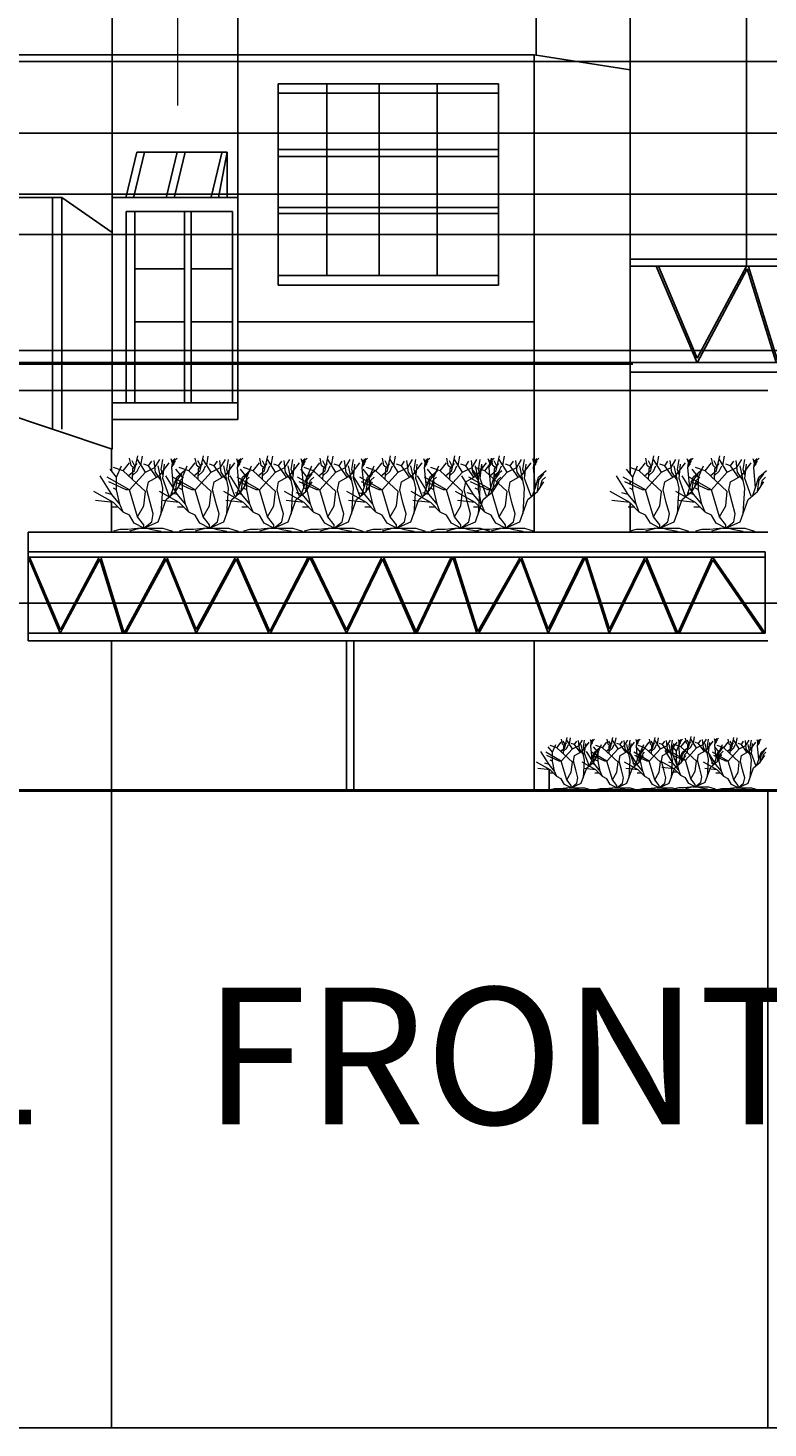
# Model space of a CAD drawing. Units: inches. Extents: x -32109 to 33221, y -19197 to 7608.
# Tile 8 of 25: x -15627 to -11787, y -5430 to 1836. Entities that reach past the tile are written whole.
import ezdxf

# ---------------------------------------------------------------- set-up
doc = ezdxf.new("R2010")
doc.units = ezdxf.units.IN
doc.header["$MEASUREMENT"] = 0
for name, color, linetype, lineweight in [('A-ANNO-DIMS', 2, 'Continuous', 18), ('A-ANNO-NOTE', 2, 'Continuous', 18), ('A-ANNO-TEXT', 7, 'Continuous', 25), ('A-ELEV', 7, 'Continuous', 25), ('L-PLNT', 3, 'Continuous', 13)]:
    doc.layers.add(name, color=color, linetype=linetype, lineweight=lineweight)
doc.styles.get("Standard").update_dxf_attribs({"font": 'arial.ttf'})
doc.dimstyles.get("Standard").update_dxf_attribs({"dimtxt": 0.18, "dimasz": 0.18, "dimexe": 0.18, "dimexo": 0.0625, "dimgap": 0.09, "dimtad": 0, "dimtih": 1, "dimtoh": 1, "dimdec": 4, "dimzin": 0, "dimdsep": 46, "dimtxsty": 'Standard', "dimcen": 0.09, "dimadec": 0, "dimazin": 0, "dimtfac": 1, "dimtdec": 4, "dimtofl": 0, "dimtmove": 0, "dimatfit": 3, "dimfxl": 1, "dimtolj": 1, "dimtzin": 0, "dimarcsym": 0})

# ---------------------------------------------------------------- blocks, each defined once
blk = doc.blocks.new('*U3')
for p, q in [((-12.47099999999977, 19.77499999999986), (-12.89799999999991, 22.04399999999987)), ((-11.27999999999997, 19.61899999999991), (-12.10400000000004, 21.18399999999974)), ((-11.43299999999999, 18.28899999999976), (-10.45699999999988, 22.7489999999998)), ((-8.160000000000082, 17.75999999999999), (-10.55999999999994, 21.59999999999991)), ((-9.480000000000018, 19.77499999999986), (-8.991999999999962, 22.59199999999964)), ((-7.200000000000045, 19.67999999999983), (-6.240000000000009, 21.11999999999989)), ((-5.085999999999785, 17.74099999999998), (-5.512999999999919, 21.33999999999992)), ((-5.279999999999972, 19.19999999999982), (-3.840000000000145, 21.59999999999991)), ((-3.376999999999952, 18.60199999999963), (-2.887999999999919, 21.57499999999982)), ((-0.5079999999998109, 21.88799999999969), (-0.0809999999999036, 20.55799999999976)), ((-0.2029999999999745, 19.14899999999988), (0.1020000000000891, 21.33999999999992)), ((-0.0199999999999818, 20.00999999999999), (0.895999999999958, 21.10499999999979)), ((0.04099999999994, 20.71399999999994), (1.384000000000241, 22.04399999999987)), ((0.1020000000000891, 21.33999999999992), (0.8350000000000363, 21.88799999999969)), ((-16.79999999999995, 16.31999999999993), (-18.7199999999998, 18.7199999999998)), ((-14.87999999999988, 18.24000000000001), (-17.75999999999999, 19.19999999999982)), ((-16.79999999999995, 16.31999999999993), (-15.3599999999999, 19.67999999999983)), ((-14.87999999999988, 18.24000000000001), (-12.95999999999981, 20.63999999999987)), ((-8.160000000000082, 12), (-14.87999999999988, 18.24000000000001)), ((-13.32499999999982, 16.72399999999993), (-11.43299999999999, 18.28899999999976)), ((-12.95999999999981, 12.47999999999979), (-8.160000000000082, 17.75999999999999)), ((-11.67699999999991, 19.07099999999991), (-12.47099999999977, 19.77499999999986)), ((-12.04299999999989, 15.6279999999997), (-11.92099999999982, 18.83600000000001)), ((-11.98199999999997, 16.80199999999968), (-10.57899999999995, 18.05399999999986)), ((-11.92099999999982, 18.83600000000001), (-10.6400000000001, 20.40100000000007)), ((-10.57899999999995, 18.05399999999986), (-9.845999999999776, 19.69699999999966)), ((-7.200000000000045, 19.67999999999983), (-8.6400000000001, 20.15999999999985)), ((-8.160000000000082, 17.75999999999999), (-5.279999999999972, 19.19999999999982)), ((-4.799999999999954, 16.31999999999993), (-7.200000000000045, 19.67999999999983)), ((-3.376999999999952, 15.31499999999982), (-5.085999999999785, 17.81899999999973)), ((-2.880000000000109, 12.95999999999981), (-4.319999999999936, 19.67999999999983)), ((-3.840000000000145, 16.79999999999995), (-0.9600000000000363, 20.63999999999987)), ((-2.765999999999849, 16.80199999999968), (-3.376999999999952, 18.60199999999963)), ((-2.880000000000109, 15.83999999999992), (-2.40000000000009, 20.15999999999985)), ((0.3460000000000036, 13.20299999999974), (-0.2029999999999745, 19.14899999999988)), ((-0.1419999999998254, 19.38399999999979), (0.5899999999999181, 20.40100000000007)), ((1.323000000000092, 16.2539999999999), (3.642000000000052, 18.28899999999976)), ((1.440000000000054, 15.3599999999999), (2.879999999999881, 17.27999999999997)), ((-18.23999999999978, 11.03999999999996), (-21.75499999999988, 16.65499999999997)), ((-12.95999999999981, 12.47999999999979), (-19.67999999999983, 16.31999999999993)), ((-13.91999999999984, 12.47999999999979), (-19.19999999999982, 14.87999999999988)), ((-16.79999999999995, 12.47999999999979), (-17.75999999999999, 12.95999999999981)), ((-16.79999999999995, 12.47999999999979), (-16.79999999999995, 16.31999999999993)), ((-7.680000000000063, 12.47999999999979), (-7.200000000000045, 14.87999999999988)), ((-7.200000000000045, 14.87999999999988), (-3.840000000000145, 16.79999999999995)), ((-3.360000000000127, 5.279999999999972), (-2.880000000000109, 12.95999999999981)), ((-0.9600000000000363, 10.55999999999994), (-2.880000000000109, 15.83999999999992)), ((-0.4800000000000182, 10.79999999999995), (0.3460000000000036, 13.20299999999974)), ((0.3460000000000036, 13.20299999999974), (1.323000000000092, 16.2539999999999)), ((0.9600000000000363, 12), (1.440000000000054, 15.3599999999999)), ((0.9600000000000363, 12), (2.879999999999881, 14.87999999999988)), ((1.920000000000072, 13.43999999999982), (2.399999999999863, 15.3599999999999)), ((2.399999999999863, 15.3599999999999), (3.359999999999899, 16.31999999999993)), ((-17.75999999999999, 8.639999999999873), (-23.66300000000001, 11.96100000000001)), ((-17.75999999999999, 8.639999999999873), (-23.12799999999993, 9.221999999999753)), ((-18.23999999999978, 11.03999999999996), (-20.15999999999985, 11.51999999999998)), ((-15.83999999999992, 8.159999999999854), (-18.23999999999978, 11.03999999999996)), ((-14.87999999999988, 5.75999999999999), (-17.75999999999999, 8.639999999999873)), ((-15.83999999999992, 8.159999999999854), (-16.79999999999995, 12.47999999999979)), ((-12.95999999999981, 12.47999999999979), (-13.91999999999984, 12.47999999999979)), ((-10.55999999999994, 4.319999999999936), (-12.95999999999981, 12.47999999999979)), ((-8.6400000000001, 7.679999999999836), (-8.160000000000082, 12)), ((-6.720000000000027, 8.639999999999873), (-7.680000000000063, 12.47999999999979)), ((-5.75999999999999, 5.279999999999972), (-6.720000000000027, 8.639999999999873)), ((-4.319999999999936, 2.879999999999881), (-1.920000000000072, 9.599999999999909)), ((-1.920000000000072, 9.599999999999909), (0.9600000000000363, 12)), ((-16.31999999999993, 7.199999999999818), (-18.23999999999978, 7.199999999999818)), ((-14.87999999999988, 5.75999999999999), (-15.83999999999992, 8.159999999999854)), ((-12.95999999999981, 4.799999999999954), (-14.87999999999988, 5.75999999999999)), ((-11.51999999999998, 2.399999999999863), (-12.95999999999981, 4.799999999999954)), ((-10.55999999999994, 4.319999999999936), (-8.6400000000001, 7.679999999999836)), ((-8.6400000000001, 1.919999999999845), (-10.55999999999994, 4.319999999999936)), ((-6.240000000000009, 2.879999999999881), (-5.75999999999999, 5.279999999999972)), ((-15.83999999999992, 0.4799999999997909), (-17.75999999999999, 0)), ((-13.43999999999982, 0.4799999999997909), (-15.83999999999992, 0.4799999999997909)), ((-9.600000000000136, 0.959999999999809), (-13.43999999999982, 0.4799999999997909)), ((-9.600000000000136, 0.959999999999809), (-12.95999999999981, 0)), ((-8.6400000000001, 0.959999999999809), (-11.51999999999998, 2.399999999999863)), ((-9.600000000000136, 0.959999999999809), (-7.680000000000063, 0.959999999999809)), ((-8.6400000000001, 0.959999999999809), (-4.319999999999936, 2.879999999999881)), ((-8.6400000000001, 0.959999999999809), (-6.240000000000009, 2.879999999999881)), ((-8.6400000000001, 0.959999999999809), (-8.6400000000001, 1.919999999999845)), ((-8.6400000000001, 0.959999999999809), (-2.880000000000109, 0.959999999999809)), ((-7.680000000000063, 0.959999999999809), (-6.240000000000009, 0.4799999999997909)), ((-6.240000000000009, 0.4799999999997909), (-3.360000000000127, 0)), ((-2.880000000000109, 0.959999999999809), (0, 0))]:
    blk.add_line(p, q)
blk = doc.blocks.new('*D10')
at = {"layer": 'A-ANNO-DIMS', "color": 0, "lineweight": -2, "transparency": 16777216}
for p, q in [((-18512.646816, -110.179138), (-18512.646816, 5772.015489000001)), ((-18512.466816, 5771.835489), (-202.0927503703958, 5771.835489)), ((18109.136745, 5771.835489), (-201.2373206296045, 5771.835489)), ((18109.316745, -101.537382), (18109.316745, 5772.015489000001))]:
    blk.add_line(p, q, dxfattribs=at)
at = {"layer": 'A-ANNO-DIMS', "color": 0, "transparency": 16777216}
for points in [[(-18512.466816, 5771.865488999999), (-18512.466816, 5771.805489000001), (-18512.646816, 5771.835489)], [(18109.136745, 5771.865488999999), (18109.136745, 5771.805489000001), (18109.316745, 5771.835489)]]:
    blk.add_solid(points, dxfattribs=at)
at = {"layer": 'Defpoints', "color": 0, "transparency": 16777216}
for p in [(18109.316745, 5771.835489), (-18512.646816, -110.241638), (18109.316745, -101.599882)]:
    blk.add_point(p, dxfattribs=at)
at = {"layer": 'A-ANNO-DIMS', "color": 0, "transparency": 16777216, "insert": (-201.6650355000002, 5771.835489), "char_height": 0.18, "attachment_point": 5}
blk.add_mtext('\\A1;36622', dxfattribs=at)
blk = doc.blocks.new('*D11')
at = {"layer": 'A-ANNO-DIMS', "color": 0, "lineweight": -2, "transparency": 16777216}
for p, q in [((14509.612941, 1705.161904000001), (25710.64858400003, 1705.161904000003)), ((25710.46858400003, 1704.981904000003), (25710.46858400003, -209.6323674706641)), ((25710.46858400003, -2124.610567999994), (25710.46858400003, -209.9962965293272)), ((-18512.58431600001, -2124.790568000001), (25710.64858400003, -2124.790567999994))]:
    blk.add_line(p, q, dxfattribs=at)
at = {"layer": 'A-ANNO-DIMS', "color": 0, "transparency": 16777216}
for points in [[(25710.43858400003, 1704.981904000003), (25710.49858400002, 1704.981904000003), (25710.46858400003, 1705.161904000003)], [(25710.43858400003, -2124.610567999994), (25710.49858400002, -2124.610567999994), (25710.46858400003, -2124.790567999994)]]:
    blk.add_solid(points, dxfattribs=at)
at = {"layer": 'Defpoints', "color": 0, "transparency": 16777216}
for p in [(14509.550441, 1705.161904000001), (-18512.64681600001, -2124.790568000001), (25710.46858400003, -2124.790567999994)]:
    blk.add_point(p, dxfattribs=at)
at = {"layer": 'A-ANNO-DIMS', "color": 0, "transparency": 16777216, "insert": (25710.46858400002, -209.8143320000029), "char_height": 0.18, "attachment_point": 5}
blk.add_mtext('\\A1;3830', dxfattribs=at)
blk = doc.blocks.new('*D21')
at = {"layer": 'A-ANNO-DIMS', "color": 0, "lineweight": -2, "transparency": 16777216}
for p, q in [((-5532.163600000002, -1149.229573), (-24361.99565300002, -1149.229573000003)), ((-24361.81565300002, -1149.409573000004), (-24361.81565300002, -1636.828167362214)), ((-24361.81565300002, -2124.610568000004), (-24361.81565300002, -1637.191973637794)), ((-5677.141660000002, -2124.790568000001), (-24361.99565300002, -2124.790568000003))]:
    blk.add_line(p, q, dxfattribs=at)
at = {"layer": 'A-ANNO-DIMS', "color": 0, "transparency": 16777216}
for points in [[(-24361.84565300001, -1149.409573000004), (-24361.78565300002, -1149.409573000004), (-24361.81565300002, -1149.229573000003)], [(-24361.84565300001, -2124.610568000004), (-24361.78565300002, -2124.610568000004), (-24361.81565300002, -2124.790568000003)]]:
    blk.add_solid(points, dxfattribs=at)
at = {"layer": 'Defpoints', "color": 0, "transparency": 16777216}
for p in [(-24361.81565300002, -1149.229573000003), (-5532.101100000001, -1149.229573), (-5677.079160000002, -2124.790568000001)]:
    blk.add_point(p, dxfattribs=at)
at = {"layer": 'A-ANNO-DIMS', "color": 0, "transparency": 16777216, "insert": (-24361.81565300001, -1637.010070499996), "char_height": 0.18, "attachment_point": 5}
blk.add_mtext('\\A1;975.6', dxfattribs=at)
blk = doc.blocks.new('*D25')
at = {"layer": 'A-ANNO-DIMS', "color": 0, "lineweight": -2, "transparency": 16777216}
for p, q in [((-15909.074234, -2124.853068), (-15909.074234, -5429.734913)), ((-15192.599186, -2124.853068), (-15192.599186, -5429.734913)), ((-15908.894234, -5429.554913), (-15551.2303525648, -5429.554913)), ((-15192.779186, -5429.554913), (-15550.4430674352, -5429.554913))]:
    blk.add_line(p, q, dxfattribs=at)
at = {"layer": 'A-ANNO-DIMS', "color": 0, "transparency": 16777216}
for points in [[(-15908.894234, -5429.524913), (-15908.894234, -5429.584913), (-15909.074234, -5429.554913)], [(-15192.779186, -5429.524913), (-15192.779186, -5429.584913), (-15192.599186, -5429.554913)]]:
    blk.add_solid(points, dxfattribs=at)
at = {"layer": 'Defpoints', "color": 0, "transparency": 16777216}
for p in [(-15909.074234, -2124.790568), (-15192.599186, -2124.790568), (-15192.599186, -5429.554913)]:
    blk.add_point(p, dxfattribs=at)
at = {"layer": 'A-ANNO-DIMS', "color": 0, "transparency": 16777216, "insert": (-15550.83671, -5429.554913), "char_height": 0.18, "attachment_point": 5}
blk.add_mtext('\\A1;716.5', dxfattribs=at)
blk = doc.blocks.new('*D26')
at = {"layer": 'A-ANNO-DIMS', "color": 0, "lineweight": -2, "transparency": 16777216}
for p, q in [((-15192.599186, -2124.853068), (-15192.599186, -5429.734913)), ((-11787.011772, -2124.853068), (-11787.011772, -5429.734913)), ((-15192.419186, -5429.554913), (-13490.26898513915, -5429.554913)), ((-11787.191772, -5429.554913), (-13489.34197286084, -5429.554913))]:
    blk.add_line(p, q, dxfattribs=at)
at = {"layer": 'A-ANNO-DIMS', "color": 0, "transparency": 16777216}
for points in [[(-15192.419186, -5429.524913), (-15192.419186, -5429.584913), (-15192.599186, -5429.554913)], [(-11787.191772, -5429.524913), (-11787.191772, -5429.584913), (-11787.011772, -5429.554913)]]:
    blk.add_solid(points, dxfattribs=at)
at = {"layer": 'Defpoints', "color": 0, "transparency": 16777216}
for p in [(-15192.599186, -2124.790568), (-11787.011772, -2124.790568), (-11787.011772, -5429.554913)]:
    blk.add_point(p, dxfattribs=at)
at = {"layer": 'A-ANNO-DIMS', "color": 0, "transparency": 16777216, "insert": (-13489.805479, -5429.554913), "char_height": 0.18, "attachment_point": 5}
blk.add_mtext('\\A1;3405.6', dxfattribs=at)
blk = doc.blocks.new('*D27')
at = {"layer": 'A-ANNO-DIMS', "color": 0, "lineweight": -2, "transparency": 16777216}
for p, q in [((-11787.011772, -2124.853068), (-11787.011772, -5429.734913)), ((-9378.382661, -2124.853068), (-9378.382661, -5429.734913)), ((-11786.831772, -5429.554913), (-10583.16231881923, -5429.554913)), ((-9378.562661, -5429.554913), (-10582.23211418076, -5429.554913))]:
    blk.add_line(p, q, dxfattribs=at)
at = {"layer": 'A-ANNO-DIMS', "color": 0, "transparency": 16777216}
for points in [[(-11786.831772, -5429.524913), (-11786.831772, -5429.584913), (-11787.011772, -5429.554913)], [(-9378.562661, -5429.524913), (-9378.562661, -5429.584913), (-9378.382661, -5429.554913)]]:
    blk.add_solid(points, dxfattribs=at)
at = {"layer": 'Defpoints', "color": 0, "transparency": 16777216}
for p in [(-11787.011772, -2124.790568), (-9378.382661, -2124.790568), (-9378.382661, -5429.554913)]:
    blk.add_point(p, dxfattribs=at)
at = {"layer": 'A-ANNO-DIMS', "color": 0, "transparency": 16777216, "insert": (-10582.6972165, -5429.554913), "char_height": 0.18, "attachment_point": 5}
blk.add_mtext('\\A1;2408.6', dxfattribs=at)
blk = doc.blocks.new('*D32')
at = {"layer": 'A-ANNO-DIMS', "color": 0, "lineweight": -2, "transparency": 16777216}
for p, q in [((-15189.725596, 955.1505220000001), (-15189.725596, 5772.015489000001)), ((-15189.545596, 5771.835489), (-14864.27138008868, 5771.835489)), ((-14538.208774, 5771.835489), (-14863.48298991132, 5771.835489)), ((-14538.028774, 1696.582648), (-14538.028774, 5772.015489))]:
    blk.add_line(p, q, dxfattribs=at)
at = {"layer": 'A-ANNO-DIMS', "color": 0, "transparency": 16777216}
for points in [[(-15189.545596, 5771.865488999999), (-15189.545596, 5771.805489000001), (-15189.725596, 5771.835489)], [(-14538.208774, 5771.865488999999), (-14538.208774, 5771.805489000001), (-14538.028774, 5771.835489)]]:
    blk.add_solid(points, dxfattribs=at)
at = {"layer": 'Defpoints', "color": 0, "transparency": 16777216}
for p in [(-14538.028774, 5771.835489), (-14538.028774, 1696.520148), (-15189.725596, 955.0880219999999)]:
    blk.add_point(p, dxfattribs=at)
at = {"layer": 'A-ANNO-DIMS', "color": 0, "transparency": 16777216, "insert": (-14863.877185, 5771.835489), "char_height": 0.18, "attachment_point": 5}
blk.add_mtext('\\A1;651.7', dxfattribs=at)
blk = doc.blocks.new('*D33')
at = {"layer": 'A-ANNO-DIMS', "color": 0, "lineweight": -2, "transparency": 16777216}
for p, q in [((-14538.028774, 1696.582648), (-14538.028774, 5772.015489)), ((-14537.848774, 5771.835489), (-13764.73509669645, 5771.835489)), ((-12990.709755, 5771.835489), (-13763.82343230355, 5771.835489)), ((-12990.529755, 1696.242222), (-12990.529755, 5772.015489000001))]:
    blk.add_line(p, q, dxfattribs=at)
at = {"layer": 'A-ANNO-DIMS', "color": 0, "transparency": 16777216}
for points in [[(-14537.848774, 5771.865488999999), (-14537.848774, 5771.805489000001), (-14538.028774, 5771.835489)], [(-12990.709755, 5771.865488999999), (-12990.709755, 5771.805489000001), (-12990.529755, 5771.835489)]]:
    blk.add_solid(points, dxfattribs=at)
at = {"layer": 'Defpoints', "color": 0, "transparency": 16777216}
for p in [(-12990.529755, 5771.835489), (-14538.028774, 1696.520148), (-12990.529755, 1696.179722)]:
    blk.add_point(p, dxfattribs=at)
at = {"layer": 'A-ANNO-DIMS', "color": 0, "transparency": 16777216, "insert": (-13764.2792645, 5771.835489), "char_height": 0.18, "attachment_point": 5}
blk.add_mtext('\\A1;1547.5', dxfattribs=at)
blk = doc.blocks.new('*D34')
at = {"layer": 'A-ANNO-DIMS', "color": 0, "lineweight": -2, "transparency": 16777216}
for p, q in [((-12990.529755, 1696.242222), (-12990.529755, 5772.015489000001)), ((-12990.349755, 5771.835489), (-12746.34064218417, 5771.835489)), ((-12501.538719, 5771.835489), (-12745.54783181582, 5771.835489)), ((-12501.358719, 1617.788543), (-12501.358719, 5772.015489000001))]:
    blk.add_line(p, q, dxfattribs=at)
at = {"layer": 'A-ANNO-DIMS', "color": 0, "transparency": 16777216}
for points in [[(-12990.349755, 5771.865488999999), (-12990.349755, 5771.805489000001), (-12990.529755, 5771.835489)], [(-12501.538719, 5771.865488999999), (-12501.538719, 5771.805489000001), (-12501.358719, 5771.835489)]]:
    blk.add_solid(points, dxfattribs=at)
at = {"layer": 'Defpoints', "color": 0, "transparency": 16777216}
for p in [(-12501.358719, 5771.835489), (-12990.529755, 1696.179722), (-12501.358719, 1617.726043)]:
    blk.add_point(p, dxfattribs=at)
at = {"layer": 'A-ANNO-DIMS', "color": 0, "transparency": 16777216, "insert": (-12745.944237, 5771.835489), "char_height": 0.18, "attachment_point": 5}
blk.add_mtext('\\A1;489.2', dxfattribs=at)
blk = doc.blocks.new('*D37')
at = {"layer": 'A-ANNO-DIMS', "color": 0, "lineweight": -2, "transparency": 16777216}
for p, q in [((-14538.09127400001, 1696.520148000001), (-24361.99565300002, 1696.520147999999)), ((-24361.81565300002, 1696.340147999999), (-24361.81565300002, -213.9532454706702)), ((-24361.81565300002, -2124.610568000003), (-24361.81565300002, -214.3171745293332)), ((-15192.66168600001, -2124.790568000001), (-24361.99565300002, -2124.790568000003))]:
    blk.add_line(p, q, dxfattribs=at)
at = {"layer": 'A-ANNO-DIMS', "color": 0, "transparency": 16777216}
for points in [[(-24361.84565300001, 1696.340147999999), (-24361.78565300002, 1696.340147999999), (-24361.81565300002, 1696.520147999999)], [(-24361.84565300001, -2124.610568000003), (-24361.78565300002, -2124.610568000003), (-24361.81565300002, -2124.790568000003)]]:
    blk.add_solid(points, dxfattribs=at)
at = {"layer": 'Defpoints', "color": 0, "transparency": 16777216}
for p in [(-14538.02877400001, 1696.520148000001), (-24361.81565300002, -2124.790568000003), (-15192.599186, -2124.790568000001)]:
    blk.add_point(p, dxfattribs=at)
at = {"layer": 'A-ANNO-DIMS', "color": 0, "transparency": 16777216, "insert": (-24361.81565300001, -214.1352099999948), "char_height": 0.18, "attachment_point": 5}
blk.add_mtext('\\A1;3821', dxfattribs=at)
blk = doc.blocks.new('*D38')
at = {"layer": 'A-ANNO-DIMS', "color": 0, "lineweight": -2, "transparency": 16777216}
for p, q in [((-11787.074272, -45.54407500000001), (-24361.99565300002, -45.54407500000204)), ((-24361.81565300002, -45.72407500000204), (-24361.81565300002, -1084.985418362212)), ((-24361.81565300002, -2124.610568000003), (-24361.81565300002, -1085.349224637792)), ((-11787.074272, -2124.790568000001), (-24361.99565300002, -2124.790568000003))]:
    blk.add_line(p, q, dxfattribs=at)
at = {"layer": 'A-ANNO-DIMS', "color": 0, "transparency": 16777216}
for points in [[(-24361.84565300001, -45.72407500000204), (-24361.78565300002, -45.72407500000204), (-24361.81565300002, -45.54407500000204)], [(-24361.84565300001, -2124.610568000003), (-24361.78565300002, -2124.610568000003), (-24361.81565300002, -2124.790568000003)]]:
    blk.add_solid(points, dxfattribs=at)
at = {"layer": 'Defpoints', "color": 0, "transparency": 16777216}
for p in [(-11787.011772, -45.54407500000001), (-24361.81565300002, -2124.790568000003), (-11787.011772, -2124.790568000001)]:
    blk.add_point(p, dxfattribs=at)
at = {"layer": 'A-ANNO-DIMS', "color": 0, "transparency": 16777216, "insert": (-24361.81565300001, -1085.167321499995), "char_height": 0.18, "attachment_point": 5}
blk.add_mtext('\\A1;2079.2', dxfattribs=at)
blk = doc.blocks.new('*D39')
at = {"layer": 'A-ANNO-DIMS', "color": 0, "lineweight": -2, "transparency": 16777216}
for p, q in [((-7375.940118000004, 1290.029218), (-24361.99565300002, 1290.029217999997)), ((-24361.81565300002, 1289.849217999998), (-24361.81565300002, -414.0189259706716)), ((-24361.81565300002, -2118.250999000004), (-24361.81565300002, -414.3828550293346)), ((-7754.474858000003, -2118.430999000001), (-24361.99565300002, -2118.430999000004))]:
    blk.add_line(p, q, dxfattribs=at)
at = {"layer": 'A-ANNO-DIMS', "color": 0, "transparency": 16777216}
for points in [[(-24361.84565300001, 1289.849217999998), (-24361.78565300002, 1289.849217999998), (-24361.81565300002, 1290.029217999997)], [(-24361.84565300001, -2118.250999000004), (-24361.78565300002, -2118.250999000004), (-24361.81565300002, -2118.430999000004)]]:
    blk.add_solid(points, dxfattribs=at)
at = {"layer": 'Defpoints', "color": 0, "transparency": 16777216}
for p in [(-7375.877618000004, 1290.029218), (-24361.81565300002, -2118.430999000004), (-7754.412358000003, -2118.430999000001)]:
    blk.add_point(p, dxfattribs=at)
at = {"layer": 'A-ANNO-DIMS', "color": 0, "transparency": 16777216, "insert": (-24361.81565300001, -414.2008904999961), "char_height": 0.18, "attachment_point": 5}
blk.add_mtext('\\A1;3408.5', dxfattribs=at)
blk = doc.blocks.new('*D40')
at = {"layer": 'A-ANNO-DIMS', "color": 0, "lineweight": -2, "transparency": 16777216}
for p, q in [((-5445.086779000002, 973.0114150000005), (-24361.99565300002, 973.0114149999976)), ((-24361.81565300002, 972.8314149999974), (-24361.81565300002, -575.7076119706716)), ((-24361.81565300002, -2124.610568000004), (-24361.81565300002, -576.0715410293345)), ((-5677.141660000002, -2124.790568000001), (-24361.99565300002, -2124.790568000003))]:
    blk.add_line(p, q, dxfattribs=at)
at = {"layer": 'A-ANNO-DIMS', "color": 0, "transparency": 16777216}
for points in [[(-24361.84565300001, 972.8314149999974), (-24361.78565300002, 972.8314149999974), (-24361.81565300002, 973.0114149999976)], [(-24361.84565300001, -2124.610568000004), (-24361.78565300002, -2124.610568000004), (-24361.81565300002, -2124.790568000003)]]:
    blk.add_solid(points, dxfattribs=at)
at = {"layer": 'Defpoints', "color": 0, "transparency": 16777216}
for p in [(-5445.024279000001, 973.0114150000005), (-24361.81565300002, -2124.790568000003), (-5677.079160000002, -2124.790568000001)]:
    blk.add_point(p, dxfattribs=at)
at = {"layer": 'A-ANNO-DIMS', "color": 0, "transparency": 16777216, "insert": (-24361.81565300001, -575.889576499996), "char_height": 0.18, "attachment_point": 5}
blk.add_mtext('\\A1;3098', dxfattribs=at)
blk = doc.blocks.new('*D41')
at = {"layer": 'A-ANNO-DIMS', "color": 0, "lineweight": -2, "transparency": 16777216}
for p, q in [((-651.0217760000003, 162.185712), (-24361.99565300002, 162.1857119999962)), ((-24361.81565300002, 162.0057119999962), (-24361.81565300002, -981.1205248622146)), ((-24361.81565300002, -2124.610568000005), (-24361.81565300002, -981.4843311377945)), ((-651.0217760000003, -2124.790568000001), (-24361.99565300002, -2124.790568000005))]:
    blk.add_line(p, q, dxfattribs=at)
at = {"layer": 'A-ANNO-DIMS', "color": 0, "transparency": 16777216}
for points in [[(-24361.84565300001, 162.0057119999962), (-24361.78565300002, 162.0057119999962), (-24361.81565300002, 162.1857119999962)], [(-24361.84565300001, -2124.610568000005), (-24361.78565300002, -2124.610568000005), (-24361.81565300002, -2124.790568000005)]]:
    blk.add_solid(points, dxfattribs=at)
at = {"layer": 'Defpoints', "color": 0, "transparency": 16777216}
for p in [(-650.9592760000002, 162.185712), (-24361.81565300002, -2124.790568000005), (-650.9592760000002, -2124.790568000001)]:
    blk.add_point(p, dxfattribs=at)
at = {"layer": 'A-ANNO-DIMS', "color": 0, "transparency": 16777216, "insert": (-24361.81565300001, -981.3024279999973), "char_height": 0.18, "attachment_point": 5}
blk.add_mtext('\\A1;2287', dxfattribs=at)
blk = doc.blocks.new('*D42')
at = {"layer": 'A-ANNO-DIMS', "color": 0, "lineweight": -2, "transparency": 16777216}
for p, q in [((-12501.42121900001, 764.1865930000002), (-24361.99565300002, 764.1865929999982)), ((-24361.81565300002, 764.0065929999982), (-24361.81565300002, 428.0747211377882)), ((-24361.81565300002, 91.77904299999811), (-24361.81565300002, 427.7109148622083)), ((-12488.224911, 91.59904300000002), (-24361.99565300002, 91.5990429999981))]:
    blk.add_line(p, q, dxfattribs=at)
at = {"layer": 'A-ANNO-DIMS', "color": 0, "transparency": 16777216}
for points in [[(-24361.84565300001, 764.0065929999982), (-24361.78565300002, 764.0065929999982), (-24361.81565300002, 764.1865929999982)], [(-24361.84565300001, 91.77904299999811), (-24361.78565300002, 91.77904299999811), (-24361.81565300002, 91.5990429999981)]]:
    blk.add_solid(points, dxfattribs=at)
at = {"layer": 'Defpoints', "color": 0, "transparency": 16777216}
for p in [(-12501.35871900001, 764.1865930000002), (-24361.81565300002, 91.5990429999981), (-12488.16241100001, 91.59904300000002)]:
    blk.add_point(p, dxfattribs=at)
at = {"layer": 'A-ANNO-DIMS', "color": 0, "transparency": 16777216, "insert": (-24361.81565300001, 427.892818000005), "char_height": 0.18, "attachment_point": 5}
blk.add_mtext('\\A1;672.6', dxfattribs=at)
blk = doc.blocks.new('*D43')
at = {"layer": 'A-ANNO-DIMS', "color": 0, "lineweight": -2, "transparency": 16777216}
for p, q in [((-7375.940118000004, 99.10345500000005), (-24361.99565300002, 99.10345499999731)), ((-24361.81565300002, 98.9234549999973), (-24361.81565300002, -1009.481868862213)), ((-24361.81565300002, -2118.250999000004), (-24361.81565300002, -1009.845675137793)), ((-7754.474858000003, -2118.430999000001), (-24361.99565300002, -2118.430999000004))]:
    blk.add_line(p, q, dxfattribs=at)
at = {"layer": 'A-ANNO-DIMS', "color": 0, "transparency": 16777216}
for points in [[(-24361.84565300001, 98.9234549999973), (-24361.78565300002, 98.9234549999973), (-24361.81565300002, 99.10345499999731)], [(-24361.84565300001, -2118.250999000004), (-24361.78565300002, -2118.250999000004), (-24361.81565300002, -2118.430999000004)]]:
    blk.add_solid(points, dxfattribs=at)
at = {"layer": 'Defpoints', "color": 0, "transparency": 16777216}
for p in [(-7375.877618000004, 99.10345500000005), (-24361.81565300002, -2118.430999000004), (-7754.412358000003, -2118.430999000001)]:
    blk.add_point(p, dxfattribs=at)
at = {"layer": 'A-ANNO-DIMS', "color": 0, "transparency": 16777216, "insert": (-24361.81565300001, -1009.663771999996), "char_height": 0.18, "attachment_point": 5}
blk.add_mtext('\\A1;2217.5', dxfattribs=at)
blk = doc.blocks.new('*D44')
at = {"layer": 'A-ANNO-DIMS', "color": 0, "lineweight": -2, "transparency": 16777216}
for p, q in [((-12501.358719, 764.249093), (-12501.358719, 5772.015489000001)), ((-12501.178719, 5771.835489), (-9938.977615976126, 5771.835489)), ((-7376.057618000001, 5771.835489), (-9938.258721023878, 5771.835489)), ((-7375.877618000001, 764.249093), (-7375.877618000001, 5772.015489000001))]:
    blk.add_line(p, q, dxfattribs=at)
at = {"layer": 'A-ANNO-DIMS', "color": 0, "transparency": 16777216}
for points in [[(-12501.178719, 5771.865488999999), (-12501.178719, 5771.805489000001), (-12501.358719, 5771.835489)], [(-7376.057618000001, 5771.865488999999), (-7376.057618000001, 5771.805489000001), (-7375.877618000001, 5771.835489)]]:
    blk.add_solid(points, dxfattribs=at)
at = {"layer": 'Defpoints', "color": 0, "transparency": 16777216}
for p in [(-7375.877618000001, 5771.835489), (-12501.358719, 764.186593), (-7375.877618000001, 764.186593)]:
    blk.add_point(p, dxfattribs=at)
at = {"layer": 'A-ANNO-DIMS', "color": 0, "transparency": 16777216, "insert": (-9938.618168500001, 5771.835489), "char_height": 0.18, "attachment_point": 5}
blk.add_mtext('\\A1;5125', dxfattribs=at)
blk = doc.blocks.new('*D45')
at = {"layer": 'A-ANNO-DIMS', "color": 0, "lineweight": -2, "transparency": 16777216}
for p, q in [((-11898.560127, 598.986194), (-11898.560127, 5772.015489000001)), ((-11898.380127, 5771.835489), (-11444.88544065006, 5771.835489)), ((-10990.638094, 5771.835489), (-11444.13278034993, 5771.835489)), ((-10990.458094, 598.060066), (-10990.458094, 5772.015489000001))]:
    blk.add_line(p, q, dxfattribs=at)
at = {"layer": 'A-ANNO-DIMS', "color": 0, "transparency": 16777216}
for points in [[(-11898.380127, 5771.865488999999), (-11898.380127, 5771.805489000001), (-11898.560127, 5771.835489)], [(-10990.638094, 5771.865488999999), (-10990.638094, 5771.805489000001), (-10990.458094, 5771.835489)]]:
    blk.add_solid(points, dxfattribs=at)
at = {"layer": 'Defpoints', "color": 0, "transparency": 16777216}
for p in [(-10990.458094, 5771.835489), (-11898.560127, 598.923694), (-10990.458094, 597.997566)]:
    blk.add_point(p, dxfattribs=at)
at = {"layer": 'A-ANNO-DIMS', "color": 0, "transparency": 16777216, "insert": (-11444.5091105, 5771.835489), "char_height": 0.18, "attachment_point": 5}
blk.add_mtext('\\A1;908.1', dxfattribs=at)
blk = doc.blocks.new('*D158')
at = {"layer": 'A-ANNO-DIMS', "color": 0, "lineweight": -2, "transparency": 16777216}
for p, q in [((5447.266114000002, 1662.169531000001), (-24361.99565300002, 1662.169530999996)), ((-24361.81565300002, 1661.989530999996), (-24361.81565300002, -230.1077594706735)), ((-24361.81565300002, -2122.568979000006), (-24361.81565300002, -230.4716885293365)), ((5279.201554000002, -2122.748979000001), (-24361.99565300002, -2122.748979000006))]:
    blk.add_line(p, q, dxfattribs=at)
at = {"layer": 'A-ANNO-DIMS', "color": 0, "transparency": 16777216}
for points in [[(-24361.84565300001, 1661.989530999996), (-24361.78565300002, 1661.989530999996), (-24361.81565300002, 1662.169530999996)], [(-24361.84565300001, -2122.568979000006), (-24361.78565300002, -2122.568979000006), (-24361.81565300002, -2122.748979000006)]]:
    blk.add_solid(points, dxfattribs=at)
at = {"layer": 'Defpoints', "color": 0, "transparency": 16777216}
for p in [(5447.328614000002, 1662.169531000001), (-24361.81565300002, -2122.748979000006), (5279.264054000002, -2122.748979000001)]:
    blk.add_point(p, dxfattribs=at)
at = {"layer": 'A-ANNO-DIMS', "color": 0, "transparency": 16777216, "insert": (-24361.81565300001, -230.289723999998), "char_height": 0.18, "attachment_point": 5}
blk.add_mtext('\\A1;3784.9', dxfattribs=at)

msp = doc.modelspace()

# ---------------------------------------------------------------- linework, layer by layer
at = {"layer": 'A-ANNO-NOTE'}
msp.add_line((-14849.34723911481, 1433.587928212481), (-14849.34723911481, 3321.835488633428), dxfattribs=at)
at = {"layer": 'A-ELEV'}
for p, q in [((-14538.02877446177, 1696.520147841968), (-12999.97204841015, 1696.520147841968)), ((-14538.02877446177, 310.5759287970213), (-14538.02877446177, 1696.520147841968)), ((-12999.97204841015, 1696.520147841968), (-12999.97204841015, 310.5759287970195)), ((-12501.35871854456, 1617.726042799927), (-12999.97204841015, 1696.520147841968)), ((-12501.35871854456, -478.3988447183314), (-12501.35871854456, 1617.726042799927)), ((-14329.08362112796, 1545.924980781834), (-13184.45012166377, 1545.924980781834)), ((-14329.08362112796, 500.3790826422248), (-14329.08362112796, 1545.924980781834)), ((-14075.81024272306, 550.7036000561241), (-14075.81024272306, 1545.924980781834)), ((-13804.33715639036, 550.7036000561241), (-13804.33715639036, 1545.924980781834)), ((-13503.62880066211, 550.7036000561241), (-13503.62880066211, 1545.924980781834)), ((-13184.45012166377, 1545.924980781834), (-13184.45012166377, 500.3790826422248)), ((-14329.08362112796, 1497.042222933355), (-13184.45012166377, 1497.042222933355)), ((-15117.21620385884, 960.9185120626353), (-15062.01029205276, 1190.667005912633)), ((-15076.8215612832, 960.9185120626353), (-15021.61564947711, 1190.667005912633)), ((-15062.01029205276, 1190.667005912633), (-14592.76116348361, 1190.667005912633)), ((-14907.26861260109, 960.9185120626353), (-14852.06270079501, 1190.667005912633)), ((-14866.87397002545, 960.9185120626353), (-14811.66805821936, 1190.667005912633)), ((-14675.75811673736, 958.0366412526345), (-14620.55220493127, 1187.785135102633)), ((-14592.76116348361, 1190.667005912633), (-14638.89296048907, 955.0880217890953)), ((-14592.76116348361, 1190.667005912633), (-14592.76116348361, 955.0880217890954)), ((-14329.08362112796, 1205.714603258725), (-13184.45012166377, 1205.714603258725)), ((-14329.08362112796, 1168.442049726963), (-13184.45012166377, 1168.442049726963)), ((-15450.80606197804, 955.0880217890953), (-17113.15498428035, 955.0880217890954)), ((-15500.14966691166, -246.6613977921091), (-15500.14966691166, 955.0880217890954)), ((-15450.80606197804, -246.6613977921091), (-15450.80606197804, 955.0880217890954)), ((-15450.80606197804, 955.0880217890954), (-15189.72559618458, 773.5367042418161)), ((-15189.72559618458, 955.0880217890954), (-15189.72559618458, -110.241637869025)), ((-15189.72559618458, 955.0880217890954), (-14912.88051272701, 955.0880217890953)), ((-14912.88051272702, 955.0880217890954), (-14538.02877446177, 955.0880217890954)), ((-15117.30845327629, -110.241637869025), (-15117.30845327628, 882.441508881311)), ((-15117.30845327628, 882.441508881311), (-14564.69062781159, 882.4415088813113)), ((-15071.95651643613, -110.241637869025), (-15071.95651643612, 882.441508881311)), ((-14814.90957782566, -110.241637869025), (-14814.90957782565, 882.441508881311)), ((-14780.77808009862, -110.241637869025), (-14780.77808009862, 882.441508881311)), ((-14564.69062781159, -110.241637869025), (-14564.69062781159, 882.441508881311)), ((-14329.08362112796, 904.792951978025), (-13184.45012166377, 904.7929519780248)), ((-14329.08362112796, 872.1794442951921), (-13184.45012166377, 872.1794442951917)), ((-7375.877618313963, 764.1865932254732), (-12501.35871854456, 764.1865932254732)), ((-15071.95651643612, 585.0279827673075), (-14814.90957782566, 585.0279827673075)), ((-14780.77808009862, 585.0279827673075), (-14564.69062781159, 585.0279827673075)), ((-12501.35871854456, 635.2624632785883), (-7375.877618313963, 635.2624632785883)), ((-7375.877618313963, 598.9236941445416), (-12501.35871854456, 598.9236941445414)), ((-12366.60595609747, 598.9236941445414), (-12366.60595609747, 599.0968064895083)), ((-12154.72056890667, 98.75487584107032), (-12366.60595609747, 599.0968064895069)), ((-12153.67122577806, 121.9209164320282), (-12355.67292113011, 598.9236941445414)), ((-11894.23986479771, 585.7976585907181), (-12154.72056890667, 98.75487584107032)), ((-11898.56012712053, 598.9236941445414), (-12153.67122577807, 121.92091643203)), ((-11745.21252362304, 99.10345488926394), (-11894.23986479771, 585.7976585907172)), ((-11734.6627692064, 98.8047831514268), (-11887.58926156124, 598.2328534291883)), ((-14329.08362112796, 550.7036000561241), (-13184.45012166377, 550.703600056124)), ((-13184.45012166377, 500.3790826422248), (-14329.08362112796, 500.3790826422248)), ((-15071.95651643612, 310.3799816166283), (-14814.90957782566, 310.3799816166284)), ((-14780.77808009862, 310.3799816166284), (-14564.69062781159, 310.3799816166283)), ((-12999.97204841015, 310.5759287970195), (-14538.02877446177, 310.5759287970195)), ((-14538.02877446177, -110.241637869025), (-14538.02877446177, 310.5759287970195)), ((-12999.97204841015, 310.5759287970195), (-13141.73192595492, 310.5759287970195)), ((-12999.97204841015, -110.241637869025), (-12999.97204841015, 310.5759287970195)), ((-12501.35871854456, 99.10345488926394), (-7375.877618313963, 99.10345488926394)), ((-7375.877618313963, 49.15697676116543), (-12501.35871854456, 49.15697676116543)), ((-15909.07423393536, -110.241637869025), (-15189.72559618458, -350.2207840895844)), ((-15189.72559618458, -110.241637869025), (-15189.72559618458, -350.2207840895844)), ((-15189.72559618458, -110.241637869025), (-14538.02877446177, -110.241637869025)), ((-14538.02877446177, -110.241637869025), (-14538.02877446177, -195.3004006951378)), ((-12999.97204841015, -110.241637869025), (-12999.97204841015, -780.5276966023393)), ((-15189.72559618458, -195.3004006951378), (-14538.02877446177, -195.3004006951378)), ((-15192.59918596467, -349.2621367997636), (-15192.59918596467, -462.2764838785319)), ((-12501.35871854456, -532.4672496993903), (-12501.35871854456, -515.6815490831111)), ((-15192.59918596467, -583.7789471828592), (-15192.59918596467, -585.486496865363)), ((-15192.59918596467, -621.7757397579829), (-15192.59918596467, -780.5276966023384)), ((-12501.35871854456, -780.5276966023393), (-12501.35871854456, -630.5031666540713)), ((-11787.37974359079, -780.5276966023393), (-15626.50010380029, -780.5276966023393)), ((-15626.50010380029, -780.5276966023393), (-15626.50010380029, -882.1826025678856)), ((-15626.50010380029, -882.1826025678856), (-11801.79647305204, -882.1826025678856)), ((-15626.50010380029, -910.8352229946985), (-15626.50010380029, -882.1826025678856)), ((-15459.43138579359, -1305.211467476512), (-15626.50010380029, -910.698726288022)), ((-11801.79647305204, -910.8352229946985), (-15626.50010380029, -910.8352229946985)), ((-15626.50010380029, -910.8352229946985), (-15626.50010380029, -1304.936617684001)), ((-15458.60399314717, -1286.945362606632), (-15617.8795558704, -910.8352229946985)), ((-15254.04592774982, -921.1849217708241), (-15459.43138579359, -1305.211467476512)), ((-15257.45239526179, -910.8352229946985), (-15458.60399314717, -1286.945362606631)), ((-15136.53991580584, -1304.936617684001), (-15254.04592774982, -921.184921770825)), ((-15128.22157932666, -1305.172116247667), (-15248.8020184297, -911.3799414115329)), ((-14914.26461008459, -911.4367267291282), (-15128.22157932666, -1305.172116247667)), ((-14910.42554701699, -920.8859792264147), (-15119.11979403489, -1304.936617684001)), ((-14754.26945270673, -1305.239749442682), (-14910.42554701699, -920.885979226414)), ((-14753.25596995104, -1286.786331798182), (-14905.9982125192, -910.8352229946985)), ((-14546.17309881141, -920.3449280315707), (-14754.26945270673, -1305.239749442682)), ((-14549.99510326002, -910.8352229946985), (-14753.25596995104, -1286.786331798183)), ((-14376.62871278106, -1304.936617684001), (-14546.17309881141, -920.3449280315698)), ((-14371.96612183574, -1295.966392323699), (-14541.42641292272, -911.5654622541796)), ((-14172.55414635566, -910.8352229946985), (-14371.96612183574, -1295.966392323699)), ((-14164.0214668832, -911.5043045778257), (-14367.88286232338, -1305.228790872628)), ((-13973.54314855781, -1305.187336483855), (-14164.0214668832, -911.5043045778257)), ((-13973.52472979662, -1287.121589469778), (-14155.58590207506, -910.8352229946985)), ((-13786.55972027591, -920.7291248533902), (-13973.54314855781, -1305.187336483855)), ((-13790.5157246804, -910.8352229946985), (-13973.52472979662, -1287.121589469777)), ((-13616.90992565921, -1308.303203194258), (-13786.55972027591, -920.7291248533884)), ((-13609.68674049994, -1305.14145439002), (-13782.02965030328, -911.4148095889976)), ((-13431.01557898117, -910.8352229946985), (-13616.80821899492, -1301.756841651205)), ((-13422.53602405275, -911.362341283866), (-13609.68674049994, -1305.14145439002)), ((-13297.89201989223, -1304.936617684001), (-13422.53602405275, -911.362341283866)), ((-13292.16016832008, -1296.919568478417), (-13414.4321298033, -910.8352229946985)), ((-13073.46816953699, -911.6482603390776), (-13292.16016832008, -1296.919568478419)), ((-13069.88922476314, -921.3158698353081), (-13287.6443140971, -1304.936617684001)), ((-12927.82467952787, -1305.067124291075), (-13069.88922476314, -921.3158698353074)), ((-12926.84058361075, -1285.013817068104), (-13065.36133419227, -910.8352229946985)), ((-12736.4672327296, -911.5675100677762), (-12927.82467952787, -1305.067124291075)), ((-12744.8788794048, -910.8352229946985), (-12926.84058361075, -1285.013817068105)), ((-12610.39633014567, -1305.067124291075), (-12736.4672327296, -911.5675100677762)), ((-12608.85752445805, -1284.027210866747), (-12728.42219249713, -910.8352229946985)), ((-12422.53446314957, -922.1121124039237), (-12610.39633014567, -1305.067124291075)), ((-12424.99219539638, -909.2191116908324), (-12608.85752445805, -1284.027210866748)), ((-12263.29069059128, -1304.936617684001), (-12422.53446314957, -922.1121124039227)), ((-12254.69657825989, -1305.067124291075), (-12417.91322831606, -912.6917597325927)), ((-12074.59553701456, -909.3189000454986), (-12254.69657825989, -1305.067124291075)), ((-12073.18473934841, -925.2545978711305), (-12245.97421235435, -1304.936617684001)), ((-11801.79647305204, -1304.936617684001), (-12074.59553701456, -909.3189000454986)), ((-11811.37417073532, -1304.936617684001), (-12073.18473934841, -925.2545978711305)), ((-11801.79647305204, -1304.936617684001), (-11801.79647305204, -882.1826025678856)), ((-15626.50010380029, -1304.936617684001), (-11801.79647305204, -1304.936617684001)), ((-15626.50010380029, -1344.318729779803), (-15626.50010380029, -1304.936617684001)), ((-14367.88286232338, -1305.228790872628), (-14368.01166470058, -1304.936617684001)), ((-11787.37974359079, -1344.318729779803), (-15626.50010380029, -1344.318729779803)), ((-15192.59918596467, -1344.318729779803), (-15192.59918596467, -2124.790568085176)), ((-13973.42121004977, -1344.318729779803), (-13973.42121004977, -2124.790568085177)), ((-13935.32324366868, -1344.318729779803), (-13935.32324366868, -2124.790568085177)), ((-12999.97204841015, -1344.318729779803), (-12999.97204841015, -1902.051897445059)), ((-12999.97204841015, -1902.05189744506), (-12999.97204841015, -2124.790568085177)), ((-12922.16664288414, -2012.0038931319), (-12922.16664288414, -2124.790568085176)), ((-18512.64681618521, -2124.790568085177), (1683.58803657419, -2124.790568085177))]:
    msp.add_line(p, q, dxfattribs=at)

# ---------------------------------------------------------------- block references
at = {"layer": 'L-PLNT'}
for p, xscale, yscale, zscale in [((-14877.17431738117, -775.9513398415686), 17.22355336887782, 17.22355336887782, 17.22355336887782), ((-14536.19370737409, -775.9513398415686), 17.22355336887782, 17.22355336887782, 17.22355336887782), ((-14202.12677833577, -775.9513398415686), 17.22355336887782, 17.22355336887782, 17.22355336887782), ((-13888.5471197516, -775.9513398415686), 17.22355336887782, 17.22355336887782, 17.22355336887782), ((-13565.14195785473, -775.9513398415686), 17.22355336887782, 17.22355336887782, 17.22355336887782), ((-13231.0752124089, -775.9513398415686), 17.22355336887782, 17.22355336887782, 17.22355336887782), ((-13000.0716040222, -775.9513398415686), 17.22355336887782, 17.22355336887782, 17.22355336887782), ((-12198.83173863289, -775.9513398415686), 17.22355336887782, 17.22355336887782, 17.22355336887782), ((-11857.45310977709, -775.9513398415686), 17.22355336887782, 17.22355336887782, 17.22355336887782), ((-12704.21453025843, -2118.430999141933), 11.97885450539613, 11.97885450539613, 11.97885450539613), ((-12467.46033551821, -2118.430999141933), 11.97885450539613, 11.97885450539613, 11.97885450539613), ((-12247.46254661442, -2118.430999141933), 11.97885450539613, 11.97885450539613, 11.97885450539613), ((-12060.58849141629, -2113.225783061954), 11.97885450539613, 11.97885450539613, 11.97885450539613), ((-11838.52549530084, -2118.430999141933), 11.97885450539613, 11.97885450539613, 11.97885450539613)]:
    msp.add_blockref('*U3', p, dxfattribs=dict(at, xscale=xscale, yscale=yscale, zscale=zscale))

# ---------------------------------------------------------------- texts
at = {"layer": 'A-ANNO-TEXT'}
msp.add_text('MONUMENTAL    FRONT   FACADE    ( CONCEPTUAL ONLY   NO DIMENSIONS )', height=709.7949465747753, dxfattribs=at).set_placement((-22238.10681632875, -3853.851877923695))

# ---------------------------------------------------------------- dimensions: what is measured, and where the dimension line sits
at = {"layer": 'A-ANNO-DIMS'}
for base, p1, p2, override, picture, middle in [((18109.316745, 5771.835489), (-18512.646816, -110.241638), (18109.316745, -101.599882), {"dimdec": 0, "dimlfac": 1, "dimrnd": 0, "dimzin": 0, "dimdsep": 46, "dimlunit": 2}, '*D10', (-201.6650355000002, 5771.835489)), ((-14538.028774, 5771.835489), (-15189.725596, 955.0880219999999), (-14538.028774, 1696.520148), {"dimdec": 1, "dimlfac": 1, "dimrnd": 0, "dimzin": 0, "dimdsep": 46, "dimlunit": 2}, '*D32', (-14863.877185, 5771.835489)), ((-12990.529755, 5771.835489), (-14538.028774, 1696.520148), (-12990.529755, 1696.179722), {"dimdec": 1, "dimlfac": 1, "dimrnd": 0, "dimzin": 0, "dimdsep": 46, "dimlunit": 2}, '*D33', (-13764.2792645, 5771.835489)), ((-12501.358719, 5771.835489), (-12990.529755, 1696.179722), (-12501.358719, 1617.726043), {"dimdec": 1, "dimlfac": 1, "dimrnd": 0, "dimzin": 0, "dimdsep": 46, "dimlunit": 2}, '*D34', (-12745.944237, 5771.835489)), ((-7375.877618000001, 5771.835489), (-12501.358719, 764.186593), (-7375.877618000001, 764.186593), {"dimdec": 0, "dimlfac": 1, "dimrnd": 0, "dimzin": 0, "dimdsep": 46, "dimlunit": 2}, '*D44', (-9938.618168500001, 5771.835489)), ((-10990.458094, 5771.835489), (-11898.560127, 598.923694), (-10990.458094, 597.997566), {"dimdec": 1, "dimlfac": 1, "dimrnd": 0, "dimzin": 0, "dimdsep": 46, "dimlunit": 2}, '*D45', (-11444.5091105, 5771.835489)), ((-15192.599186, -5429.554913), (-15909.074234, -2124.790568), (-15192.599186, -2124.790568), {"dimdec": 1, "dimlfac": 1, "dimrnd": 0, "dimzin": 0, "dimdsep": 46, "dimlunit": 2}, '*D25', (-15550.83671, -5429.554913)), ((-11787.011772, -5429.554913), (-15192.599186, -2124.790568), (-11787.011772, -2124.790568), {"dimdec": 1, "dimlfac": 1, "dimrnd": 0, "dimzin": 0, "dimdsep": 46, "dimlunit": 2}, '*D26', (-13489.805479, -5429.554913)), ((-9378.382661, -5429.554913), (-11787.011772, -2124.790568), (-9378.382661, -2124.790568), {"dimdec": 1, "dimlfac": 1, "dimrnd": 0, "dimzin": 0, "dimdsep": 46, "dimlunit": 2}, '*D27', (-10582.6972165, -5429.554913))]:
    dim = msp.add_linear_dim(base=base, p1=p1, p2=p2, dimstyle='Standard', override=override, dxfattribs=at)
    dim.commit()
    dim.dimension.update_dxf_attribs({"geometry": picture, "text_midpoint": middle})
for base, p1, p2, override, picture, middle in [((-24361.81565300002, -2124.790568000003), (-14538.028774, 1696.520148), (-15192.599186, -2124.790568), {"dimdec": 0, "dimlfac": 1, "dimrnd": 0, "dimzin": 0, "dimdsep": 46, "dimlunit": 2}, '*D37', (-24361.81565300001, -214.1352099999948)), ((25710.46858400003, -2124.790567999994), (14509.550441, 1705.161904), (-18512.646816, -2124.790568), {"dimdec": 0, "dimlfac": 1, "dimrnd": 0, "dimzin": 0, "dimdsep": 46, "dimlunit": 2}, '*D11', (25710.46858400002, -209.8143320000029)), ((-24361.81565300002, -2122.748979000006), (5447.328613999999, 1662.169531), (5279.264054, -2122.748979), {"dimdec": 1, "dimlfac": 1, "dimrnd": 0, "dimzin": 0, "dimdsep": 46, "dimlunit": 2}, '*D158', (-24361.81565300001, -230.289723999998)), ((-24361.81565300002, -2118.430999000004), (-7375.877618000001, 1290.029218), (-7754.412358, -2118.430999), {"dimdec": 1, "dimlfac": 1, "dimrnd": 0, "dimzin": 0, "dimdsep": 46, "dimlunit": 2}, '*D39', (-24361.81565300001, -414.2008904999961)), ((-24361.81565300002, -2124.790568000003), (-5445.024279, 973.011415), (-5677.07916, -2124.790568), {"dimdec": 0, "dimlfac": 1, "dimrnd": 0, "dimzin": 0, "dimdsep": 46, "dimlunit": 2}, '*D40', (-24361.81565300001, -575.889576499996)), ((-24361.81565300002, 91.5990429999981), (-12501.358719, 764.186593), (-12488.162411, 91.599043), {"dimdec": 1, "dimlfac": 1, "dimrnd": 0, "dimzin": 0, "dimdsep": 46, "dimlunit": 2}, '*D42', (-24361.81565300001, 427.892818000005)), ((-24361.81565300002, -2124.790568000005), (-650.959276, 162.185712), (-650.959276, -2124.790568), {"dimdec": 0, "dimlfac": 1, "dimrnd": 0, "dimzin": 0, "dimdsep": 46, "dimlunit": 2}, '*D41', (-24361.81565300001, -981.3024279999973)), ((-24361.81565300002, -2118.430999000004), (-7375.877618000001, 99.103455), (-7754.412358, -2118.430999), {"dimdec": 1, "dimlfac": 1, "dimrnd": 0, "dimzin": 0, "dimdsep": 46, "dimlunit": 2}, '*D43', (-24361.81565300001, -1009.663771999996)), ((-24361.81565300002, -2124.790568000003), (-11787.011772, -45.54407499999999), (-11787.011772, -2124.790568), {"dimdec": 1, "dimlfac": 1, "dimrnd": 0, "dimzin": 0, "dimdsep": 46, "dimlunit": 2}, '*D38', (-24361.81565300001, -1085.167321499995)), ((-24361.81565300002, -1149.229573000003), (-5677.07916, -2124.790568), (-5532.1011, -1149.229573), {"dimdec": 1, "dimlfac": 1, "dimrnd": 0, "dimzin": 0, "dimdsep": 46, "dimlunit": 2}, '*D21', (-24361.81565300001, -1637.010070499996))]:
    dim = msp.add_linear_dim(base=base, p1=p1, p2=p2, angle=90, dimstyle='Standard', override=override, dxfattribs=at)
    dim.commit()
    dim.dimension.update_dxf_attribs({"geometry": picture, "text_midpoint": middle})

doc.saveas('drawing.dxf')
